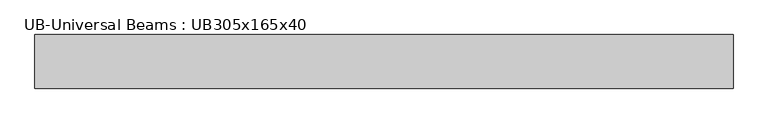
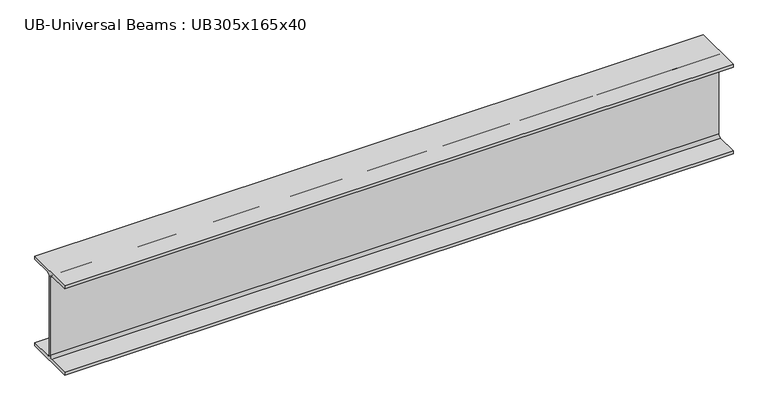
"""IFC4 building model written with IfcOpenShell, lengths in millimetres: beam geometry, UB-Universal Beams : UB305x165x40."""

from ifc_helpers import new_model, si_unit, point, frame, frame_2d, origin, place, context, project, spatial, polyline, circle_curve, trimmed, segment, composite_curve, outline, extrude, source, transform, mapped, element, save


def ub_universal_beams_ub305x165x40_d9098774(model_context):
    return source(origin(), model_context, "Body", "SweptSolid", [
        extrude(outline(composite_curve([segment(polyline([(82.5, -141.5), (82.5, -151.7), (-82.5, -151.7), (-82.5, -141.5), (-11.9, -141.5)]), True, "CONTINUOUS"), segment(trimmed(circle_curve(frame_2d((-11.9, -132.6)), 8.9), [point((-11.9, -141.5))], [point((-3.0, -132.6))], True, "CARTESIAN"), True, "CONTINUOUS"), segment(polyline([(-3.0, -132.6), (-3.0, 132.6)]), True, "CONTINUOUS"), segment(trimmed(circle_curve(frame_2d((-11.9, 132.6)), 8.9), [point((-3.0, 132.6))], [point((-11.9, 141.5))], True, "CARTESIAN"), True, "CONTINUOUS"), segment(polyline([(-11.9, 141.5), (-82.5, 141.5), (-82.5, 151.7), (82.5, 151.7), (82.5, 141.5), (11.9, 141.5)]), True, "CONTINUOUS"), segment(trimmed(circle_curve(frame_2d((11.9, 132.6)), 8.9), [point((11.9, 141.5))], [point((3.0, 132.6))], True, "CARTESIAN"), True, "CONTINUOUS"), segment(polyline([(3.0, 132.6), (3.0, -132.6)]), True, "CONTINUOUS"), segment(trimmed(circle_curve(frame_2d((11.9, -132.6)), 8.9), [point((3.0, -132.6))], [point((11.9, -141.5))], True, "CARTESIAN"), True, "CONTINUOUS"), segment(polyline([(11.9, -141.5), (82.5, -141.5)]), True, "CONTINUOUS")], self_intersect=False)), frame((-1085.6, 0.0, 0.0), z_axis=(1.0, 0.0, 0.0), x_axis=(0.0, 1.0, 0.0)), (0.0, 0.0, 1.0), 2149.0),
    ])


if __name__ == "__main__":
    model = new_model("IFC4")
    model_context = context("Model", 3, world=origin())
    ifc_project = project(units=[si_unit("LENGTHUNIT", "METRE", prefix="MILLI")], contexts=[model_context])
    site = spatial("IfcSite", under=ifc_project)
    building = spatial("IfcBuilding", under=site)
    placement = place(None, origin())
    ub_universal_beams_ub305x165x40_shape = ub_universal_beams_ub305x165x40_d9098774(model_context)
    element("IfcBeam", 1, ObjectType="UB-Universal Beams : UB305x165x40", at=placement, inside=building, context=model_context, shape_type="MappedRepresentation", body=[
        mapped(ub_universal_beams_ub305x165x40_shape, transform((0.0, 0.0, 0.0), x_axis=(1.0, 0.0, 0.0), y_axis=(0.0, 1.0, 0.0), z_axis=(0.0, 0.0, 1.0))),
    ])
    save(model, "model.ifc")

# Revit data of these elements
# Type "UB-Universal Beams : UB305x165x40"
#   Section Name Key = "UB305X165X40"
#   Width = 16.5 cm
#   Web Thickness = 0.6 cm
#   Web Fillet = 0.89 cm
#   Warping Constant = 164000.0 cm⁶
#   Torsional Moment of Inertia = 14.70 cm⁴
#   Section Area = 51.3 cm²
#   Plastic Modulus weak axis = 142.0 cm³
#   Plastic Modulus strong axis = 623.0 cm³
#   Nominal Weight = 40.2999 kgf/m
#   Moment of Inertia weak axis = 764.00 cm⁴
#   Moment of Inertia strong axis = 8503.00 cm⁴
#   Height = 30.34 cm
#   Flange Thickness = 1.02 cm
#   Elastic Modulus weak axis = 92.6 cm³
#   Elastic Modulus strong axis = 560.0 cm³
#   Centroid Vertical = 15.17 cm
#   Centroid Horizontal = 8.25 cm
#   Bolt Spacing = 9.0 cm
#   Length [instance default] = 1500 mm
#   Structural Material [instance default] = Metal - Steel 43-275
#   Type Comments = ""
#   Assembly Code = ""
# Element 1 (IfcBeam, "UB-Universal Beams : UB305x165x40")
#   Materials on its faces: "Metal - Steel 43-275"
# Materials
#   "Metal - Steel 43-275": class "Metal", colour RGB 247 247 247, transparency 0, Cost = 0
